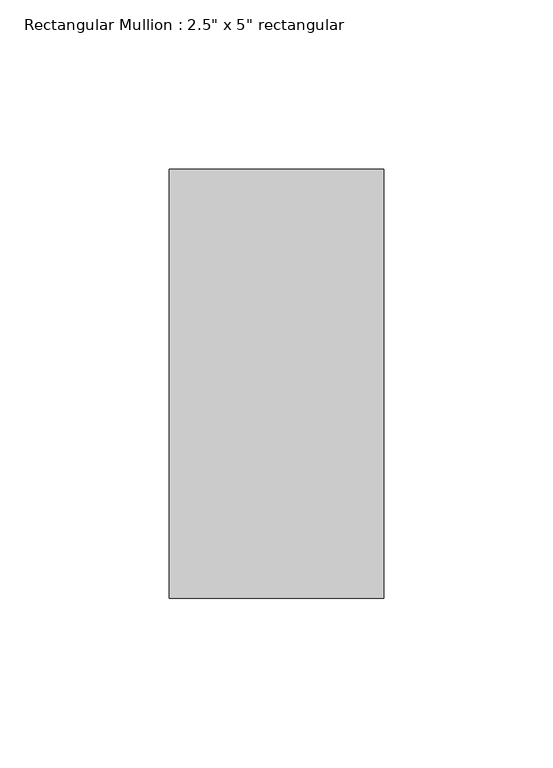
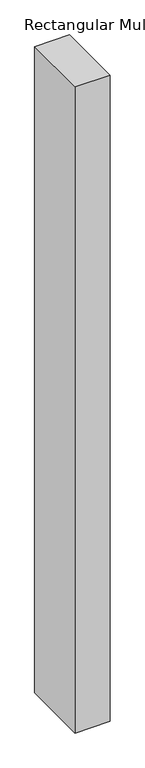
"""IFC4 building model written with IfcOpenShell, lengths in millimetres: member geometry."""

from ifc_helpers import new_model, si_unit, frame, origin, place, context, project, spatial, polyline, outline, extrude, source, transform, mapped, element, save


def member_d19d9823(model_context):
    return source(origin(), model_context, "Body", "SweptSolid", [
        extrude(outline(polyline([(31.75, 63.5), (31.75, -63.5), (-31.75, -63.5), (-31.75, 63.5), (31.75, 63.5)])), frame((0.0, 0.0, -1239.1384032), z_axis=(0.0, 0.0, 1.0), x_axis=(1.0, 0.0, 0.0)), (0.0, 0.0, 1.0), 1239.1384032),
    ])


if __name__ == "__main__":
    model = new_model("IFC4")
    model_context = context("Model", 3, world=origin())
    ifc_project = project(units=[si_unit("LENGTHUNIT", "METRE", prefix="MILLI")], contexts=[model_context])
    site = spatial("IfcSite", under=ifc_project)
    building = spatial("IfcBuilding", under=site)
    placement = place(None, origin())
    member_shape = member_d19d9823(model_context)
    element("IfcMember", 1, ObjectType="Rectangular Mullion : 2.5\" x 5\" rectangular", at=placement, inside=building, context=model_context, shape_type="MappedRepresentation", body=[
        mapped(member_shape, transform((0.0, 0.0, 0.0), x_axis=(1.0, 0.0, 0.0), y_axis=(0.0, 1.0, 0.0), z_axis=(0.0, 0.0, 1.0))),
    ])
    save(model, "model.ifc")

# Revit data of these elements
# Type "Rectangular Mullion : 2.5\" x 5\" rectangular"
#   built-in parameter 1007304 = 0.416667 (stored number, unit not read)
#   built-in parameter 1007301 = 0.104167 (stored number, unit not read)
#   built-in parameter 1007300 = 0.104167 (stored number, unit not read)
# Element 1 (IfcMember, "Rectangular Mullion : 2.5\" x 5\" rectangular")
#   Materials on its faces: "Aluminum"
# Materials
#   "Aluminum": class "Metal", colour RGB 247 247 247, transparency 0, Description = "Aluminum 6061", Cost = 0
